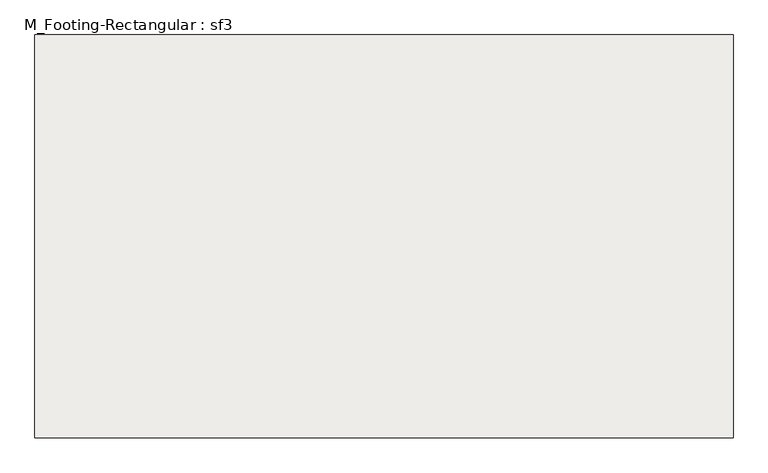
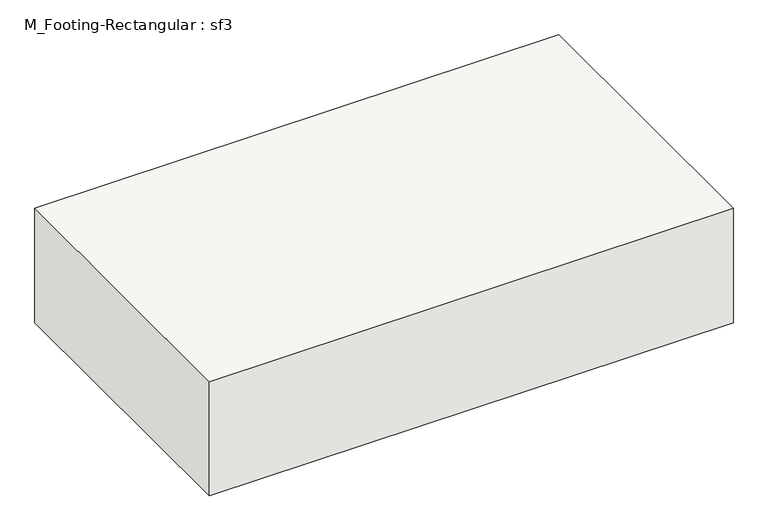
"""IFC4 building model written with IfcOpenShell, lengths in millimetres: slab geometry, M_Footing-Rectangular : sf3."""

from ifc_helpers import new_model, si_unit, frame, origin, place, context, project, spatial, polyline, outline, extrude, source, transform, mapped, element, save


def m_footing_rectangular_sf3_0b37110f(model_context):
    return source(origin(), model_context, "Body", "SweptSolid", [
        extrude(outline(polyline([(990.6, 571.5), (990.6, -571.5), (-990.6, -571.5), (-990.6, 571.5), (990.6, 571.5)])), frame((0.0, 0.0, -457.2), z_axis=(0.0, 0.0, 1.0), x_axis=(1.0, 0.0, 0.0)), (0.0, 0.0, 1.0), 457.2),
    ])


if __name__ == "__main__":
    model = new_model("IFC4")
    model_context = context("Model", 3, world=origin())
    ifc_project = project(units=[si_unit("LENGTHUNIT", "METRE", prefix="MILLI")], contexts=[model_context])
    site = spatial("IfcSite", under=ifc_project)
    building = spatial("IfcBuilding", under=site)
    placement = place(None, origin())
    m_footing_rectangular_sf3_shape = m_footing_rectangular_sf3_0b37110f(model_context)
    element("IfcSlab", 1, ObjectType="M_Footing-Rectangular : sf3", at=placement, inside=building, context=model_context, shape_type="MappedRepresentation", body=[
        mapped(m_footing_rectangular_sf3_shape, transform((0.0, 0.0, 0.0), x_axis=(1.0, 0.0, 0.0), y_axis=(0.0, 1.0, 0.0), z_axis=(0.0, 0.0, 1.0))),
    ])
    save(model, "model.ifc")

# Revit data of these elements
# Type "M_Footing-Rectangular : sf3"
#   Width = 1981.2 mm
#   Length = 1143 mm
#   Foundation Thickness = 457.2 mm
#   Structural Material [instance default] = Concrete, Cast-in-Place gray
#   Assembly Code = ""
# Element 1 (IfcSlab, "M_Footing-Rectangular : sf3")
#   Materials on its faces: "Concrete, Cast-in-Place gray"
# Materials
#   "Concrete, Cast-in-Place gray": class "Concrete", colour RGB 192 192 192, transparency 0, Description = "Cast-in-place concrete", Cost = 0
